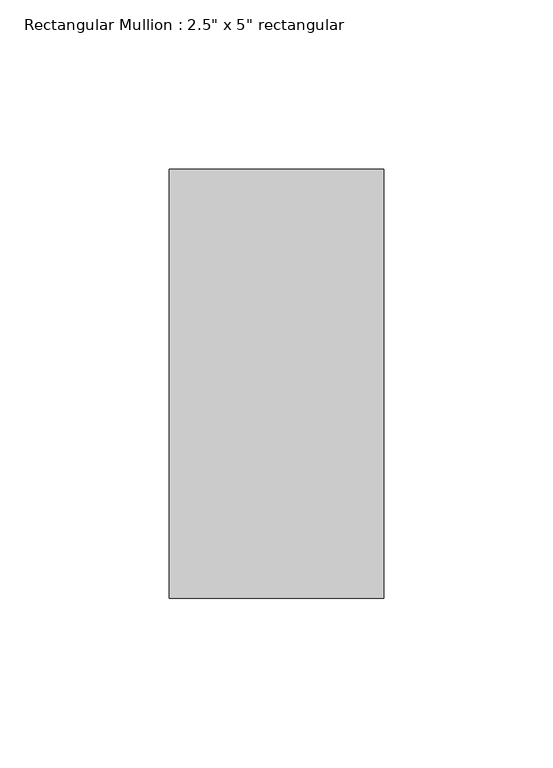
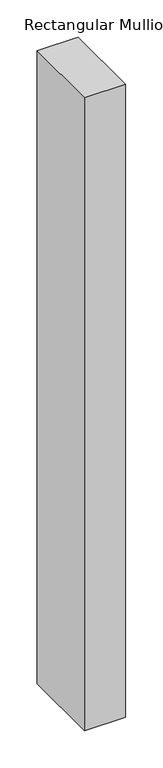
"""IFC4 building model written with IfcOpenShell, lengths in millimetres: member geometry."""

from ifc_helpers import new_model, si_unit, frame, origin, place, context, project, spatial, polyline, outline, extrude, source, transform, mapped, element, save


def member_309cb93c(model_context):
    return source(origin(), model_context, "Body", "SweptSolid", [
        extrude(outline(polyline([(31.75, 63.5), (31.75, -63.5), (-31.75, -63.5), (-31.75, 63.5), (31.75, 63.5)])), frame((0.0, 0.0, -1035.05), z_axis=(0.0, 0.0, 1.0), x_axis=(1.0, 0.0, 0.0)), (0.0, 0.0, 1.0), 1035.05),
    ])


if __name__ == "__main__":
    model = new_model("IFC4")
    model_context = context("Model", 3, world=origin())
    ifc_project = project(units=[si_unit("LENGTHUNIT", "METRE", prefix="MILLI")], contexts=[model_context])
    site = spatial("IfcSite", under=ifc_project)
    building = spatial("IfcBuilding", under=site)
    placement = place(None, origin())
    member_shape = member_309cb93c(model_context)
    element("IfcMember", 1, ObjectType="Rectangular Mullion : 2.5\" x 5\" rectangular", at=placement, inside=building, context=model_context, shape_type="MappedRepresentation", body=[
        mapped(member_shape, transform((0.0, 0.0, 0.0), x_axis=(1.0, 0.0, 0.0), y_axis=(0.0, 1.0, 0.0), z_axis=(0.0, 0.0, 1.0))),
    ])
    save(model, "model.ifc")

# Revit data of these elements
# Type "Rectangular Mullion : 2.5\" x 5\" rectangular"
#   built-in parameter 1007304 = 0.416667 (stored number, unit not read)
#   built-in parameter 1007301 = 0.104167 (stored number, unit not read)
#   built-in parameter 1007300 = 0.104167 (stored number, unit not read)
# Element 1 (IfcMember, "Rectangular Mullion : 2.5\" x 5\" rectangular")
#   Materials on its faces: "Aluminum"
# Materials
#   "Aluminum": class "Metal", colour RGB 247 247 247, transparency 0, Description = "Aluminum 6061", Cost = 0
